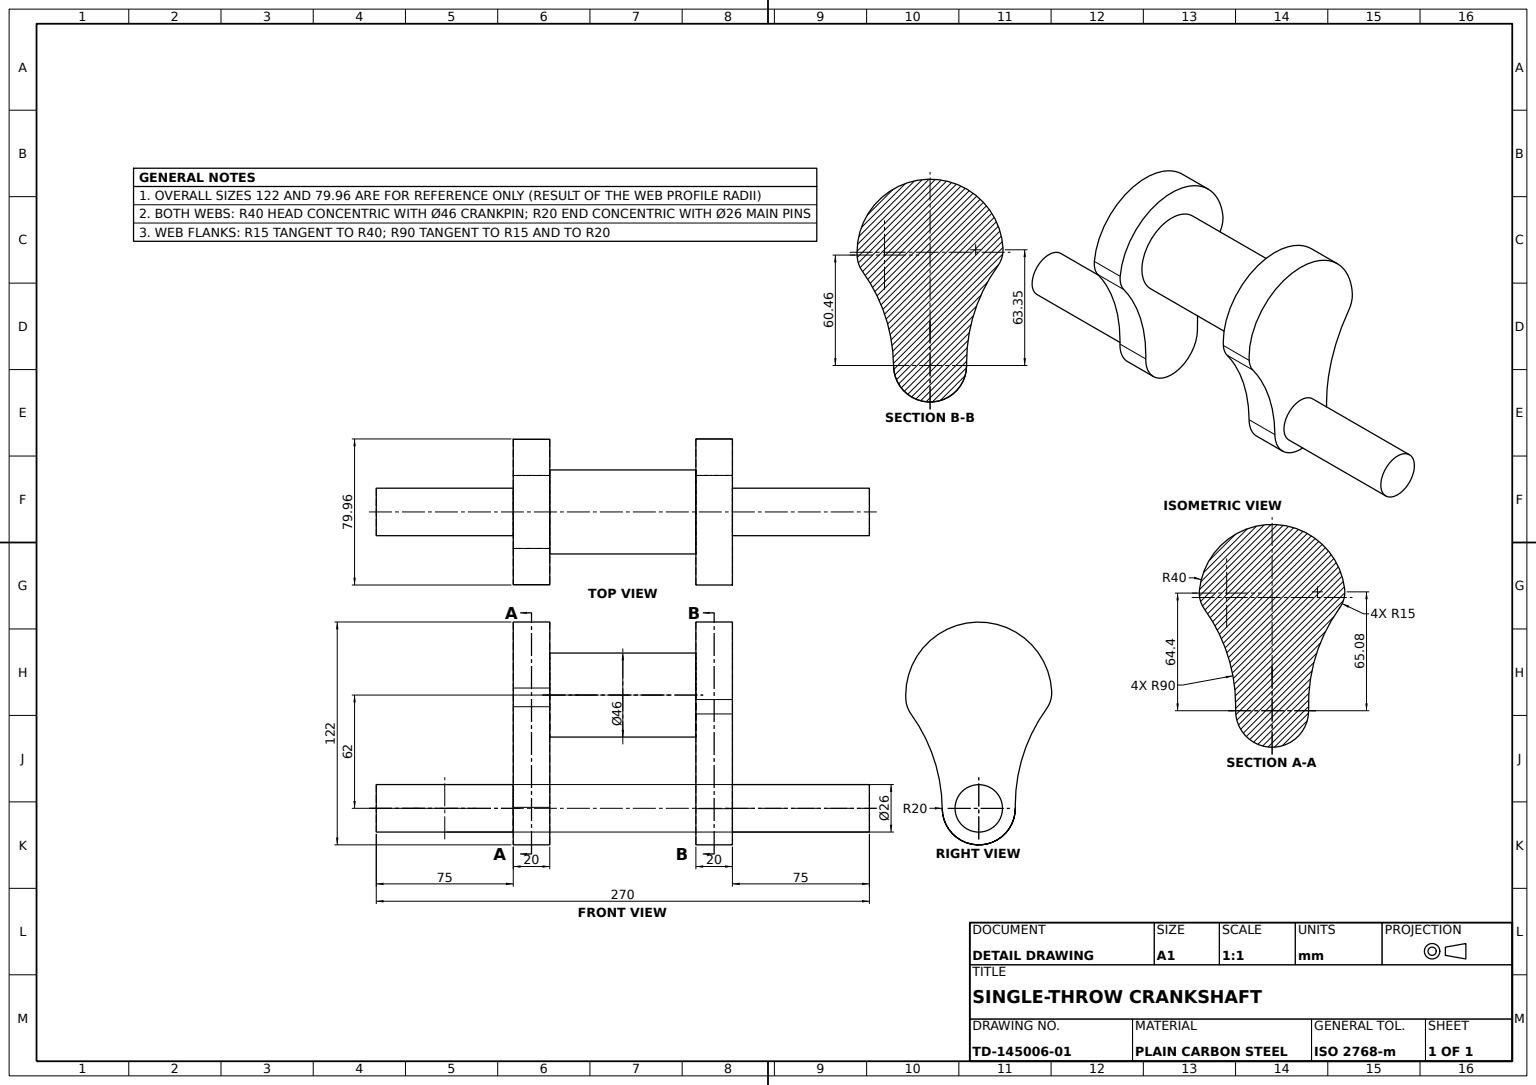
SolidWorks part; units mm, degrees
material "Plain Carbon Steel"
ref_plane "Front Plane" through (0, 0, 0) normal (0, 0, 1) x (1, 0, 0)
ref_plane "Top Plane" through (0, 0, 0) normal (0, 1, 0) x (1, 0, 0)
ref_plane "Right Plane" through (0, 0, 0) normal (1, 0, 0) x (0, 0, -1)
sketch "Front Plate Profile" plane through (0, 0, 0) normal (0, 0, 1) x (1, 0, 0)
  line L0 (0, 0) -> (0, 62) construction
  arc A0 (-19.9892, 0.6572) -> (19.9932, 0.5216) centre (0, 0) ccw
  arc A1 (39.8146, 65.8473) -> (-39.6957, 66.9244) centre (0, 62) ccw
  arc A3 (-39.6957, 66.9244) -> (-36.9714, 56.2973) centre (-24.8098, 65.0778) ccw
  arc A4 (-19.9892, 0.6572) -> (-36.9714, 56.2973) centre (-109.9406, 3.6144) ccw
  arc A5 (37.0382, 55.6137) -> (39.8146, 65.8473) centre (24.8841, 64.4045) ccw
  arc A6 (19.9932, 0.5216) -> (37.0382, 55.6137) centre (109.9626, 2.8688) cw
  dimension "D1" = 40
  dimension "D2" = 80
  dimension "D4" = 30
  dimension "D6" = 90
  dimension "D7" = 30
  dimension "D8" = 90
  dimension "D3" = 62
  dimension "D5" = 65.0778
  dimension "D9" = 64.4045
extrude "Front Plate" add sketch "Front Plate Profile" along normal blind 20
sketch "Front Pin Profile Ø26" plane through (0, 0, 20) normal (0, 0, 1) x (1, 0, 0)
  circle A0 centre (0, 0) radius 13
  dimension "D1" = 26
extrude "Front Pin Ø26" add sketch "Front Pin Profile Ø26" along normal blind 75
sketch "Journal Profile Ø46" plane through (0, 0, 0) normal (0, 0, -1) x (-1, 0, 0)
  circle A0 centre (0, 62) radius 23
  dimension "D1" = 46
extrude "Journal Ø46" add sketch "Journal Profile Ø46" along normal blind 80
ref_plane "Rear Plate Plane" through (0, 0, -80) normal (0, 0, 1) x (1, 0, 0)
sketch "Rear Plate Profile" plane through (0, 0, -80) normal (0, 0, 1) x (1, 0, 0)
  arc A0 (-19.9975, 0.3158) -> (19.999, -0.2045) centre (0, 0) ccw
  arc A1 (39.9242, 59.5392) -> (-39.9417, 64.1592) centre (0, 62) ccw
  arc A2 (37.1014, 51.6639) -> (39.9242, 59.5392) centre (24.9526, 60.462) ccw
  arc A3 (-39.9417, 64.1592) -> (-37.1097, 54.5477) centre (-24.9635, 63.3495) ccw
  arc A4 (37.1014, 51.6639) -> (19.999, -0.2045) centre (109.9942, -1.1247) ccw
  arc A5 (-19.9975, 0.3158) -> (-37.1097, 54.5477) centre (-109.9863, 1.7368) ccw
  dimension "D1" = 40
  dimension "D2" = 80
  dimension "D3" = 30
  dimension "D5" = 30
  dimension "D6" = 90
  dimension "D7" = 63.3495
  dimension "D8" = 90
  dimension "D4" = 60.462
extrude "Rear Plate" add sketch "Rear Plate Profile" against normal blind 20
sketch "Rear Pin Profile Ø26" plane through (0, 0, -100) normal (0, 0, -1) x (-1, 0, 0)
  circle A0 centre (0, 0) radius 13
  dimension "D1" = 26
extrude "Rear Pin Ø26" add sketch "Rear Pin Profile Ø26" along normal blind 75
